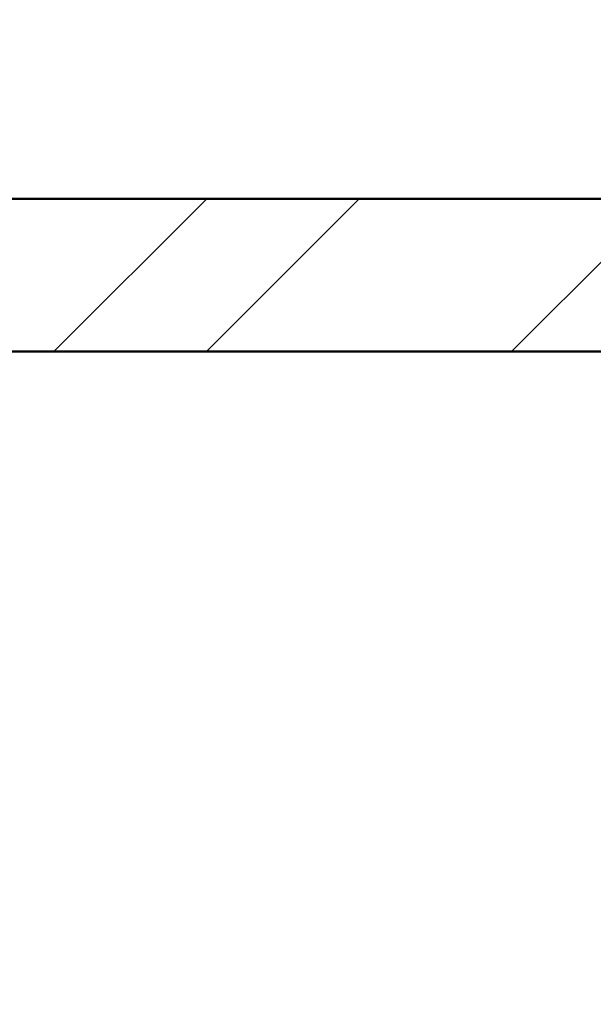
# Model space of a CAD drawing. Units: inches. Extents: x 1901 to 2863, y 888 to 2433.
# Tile 27 of 91: x 2540 to 2557, y 1376 to 1405. Entities that reach past the tile are written whole.
import ezdxf

# ---------------------------------------------------------------- set-up
doc = ezdxf.new("R2010")
doc.units = ezdxf.units.IN
doc.layers.add('A-WALL', color=7, linetype='Continuous', lineweight=50)
doc.layers.add('A-WALL-PATT', color=8, linetype='Continuous', lineweight=13)

msp = doc.modelspace()

# ---------------------------------------------------------------- hatches: boundary and pattern name
at = {"layer": 'A-WALL-PATT'}
h = msp.add_hatch(dxfattribs=at)
h.set_pattern_fill('ANSI32', color=256)
h.paths.add_polyline_path([(2443.926, 2139.888), (2439.426, 2139.888), (2439.426, 2069.348), (2441.676, 2069.348), (2443.926, 2069.348), (2443.926, 2078.634), (2521.926, 2078.634), (2521.926, 2075.067), (2524.176, 2075.067), (2526.426, 2075.067), (2526.426, 2078.634), (2571.755, 2078.634), (2571.755, 2080.884), (2571.755, 2083.134), (2443.926, 2083.134)])
h.paths.add_polyline_path([(2526.426, 2054.634), (2524.176, 2054.634), (2521.926, 2054.634), (2521.926, 2030.634), (2443.926, 2030.634), (2443.926, 2045.348), (2439.426, 2045.348), (2439.426, 1983.867), (2443.926, 1983.867), (2443.926, 2026.134), (2521.926, 2026.134), (2526.426, 2026.134)])
h.paths.add_polyline_path([(2443.926, 1923.867), (2439.426, 1923.867), (2439.426, 1872.634), (2443.926, 1872.634)])
h.paths.add_polyline_path([(2636.233, 1766.134), (2609.926, 1766.134), (2609.926, 1779.785), (2605.426, 1779.785), (2605.426, 1766.134), (2486.614, 1766.134), (2486.614, 1770.671), (2482.114, 1770.671), (2482.114, 1766.134), (2482.114, 1761.634), (2636.233, 1761.634), (2636.233, 1763.884)])
h.paths.add_polyline_path([(2519.536, 1663.384), (2519.536, 1665.634), (2494.926, 1665.634), (2481.831, 1665.634), (2481.831, 1663.384), (2481.831, 1661.134), (2490.426, 1661.134), (2490.426, 1640.157), (2494.926, 1640.157), (2494.926, 1661.134), (2519.536, 1661.134)])
h.paths.add_polyline_path([(2443.926, 1712.134), (2443.926, 1716.634), (2414.464, 1716.634), (2414.464, 1712.134), (2439.426, 1712.134), (2439.426, 1545.507), (2443.926, 1545.507), (2443.926, 1661.134), (2448.475, 1661.134), (2448.475, 1665.634), (2443.926, 1665.634)])
h.paths.add_polyline_path([(2343.426, 1712.134), (2365.525, 1712.134), (2365.525, 1714.384), (2365.525, 1716.634), (2333.871, 1716.634), (2333.871, 1714.384), (2333.871, 1712.134), (2338.926, 1712.134), (2338.926, 1575.634), (2338.926, 1545.507), (2343.426, 1545.507), (2343.426, 1547.507), (2343.426, 1580.134)])
h.paths.add_polyline_path([(2752.926, 1665.634), (2579.536, 1665.634), (2579.536, 1661.134), (2615.926, 1661.134), (2615.926, 1529.134), (2598.931, 1529.134), (2598.931, 1524.634), (2623.127, 1524.634), (2623.127, 1526.884), (2623.127, 1529.134), (2620.426, 1529.134), (2620.426, 1661.134), (2748.426, 1661.134), (2748.426, 1633.499), (2752.926, 1633.499)])
h.paths.add_polyline_path([(2752.926, 1419.929), (2748.426, 1419.929), (2748.426, 1400.134), (2659.426, 1400.134), (2659.426, 1444.333), (2657.176, 1444.333), (2654.926, 1444.333), (2654.926, 1400.134), (2643.649, 1400.134), (2643.649, 1395.634), (2748.426, 1395.634), (2748.426, 1364.035), (2752.926, 1364.035)])
h.paths.add_polyline_path([(2752.926, 1492.878), (2748.426, 1492.878), (2748.426, 1476.634), (2667.426, 1476.634), (2667.426, 1479.71), (2665.176, 1479.71), (2662.926, 1479.71), (2662.926, 1476.634), (2654.926, 1476.634), (2654.926, 1469.536), (2659.426, 1469.536), (2659.426, 1472.134), (2748.426, 1472.134), (2748.426, 1455.929), (2752.926, 1455.929)])
h.paths.add_polyline_path([(2752.926, 1304.035), (2748.426, 1304.035), (2748.426, 1263.634), (2738.66, 1263.634), (2738.66, 1259.134), (2752.926, 1259.134)])
h.paths.add_polyline_path([(2685.926, 1259.134), (2695.49, 1259.134), (2695.49, 1261.384), (2695.49, 1263.634), (2677.837, 1263.634), (2677.837, 1261.384), (2677.837, 1259.134), (2681.426, 1259.134), (2681.426, 1203.634), (2653.277, 1203.634), (2653.277, 1199.134), (2685.926, 1199.134), (2685.926, 1203.634)])
h.paths.add_polyline_path([(2609.426, 1395.634), (2611.848, 1395.634), (2611.848, 1400.134), (2598.888, 1400.134), (2598.888, 1397.884), (2598.888, 1395.634), (2604.926, 1395.634), (2604.926, 1268.134), (2554.726, 1268.134), (2554.726, 1265.884), (2554.726, 1263.634), (2604.926, 1263.634), (2604.926, 1203.634), (2571.306, 1203.634), (2571.306, 1199.134), (2604.926, 1199.134), (2629.277, 1199.134), (2629.277, 1201.384), (2629.277, 1203.634), (2609.426, 1203.634), (2609.426, 1258.634), (2609.426, 1259.134), (2654.804, 1259.134), (2654.804, 1263.634), (2609.426, 1263.634)])
h.paths.add_polyline_path([(2443.926, 1304.035), (2439.426, 1304.035), (2439.426, 1259.134), (2443.926, 1259.134), (2456.16, 1259.134), (2456.16, 1261.384), (2456.16, 1263.634), (2443.926, 1263.634)])
h.paths.add_polyline_path([(2525.426, 1263.634), (2531.778, 1263.634), (2531.778, 1268.134), (2520.926, 1268.134), (2520.926, 1263.634), (2511.409, 1263.634), (2511.409, 1259.134), (2520.926, 1259.134), (2520.926, 1199.134), (2547.306, 1199.134), (2547.306, 1201.384), (2547.306, 1203.634), (2525.426, 1203.634)])
h.paths.add_polyline_path([(2443.926, 1434.842), (2439.426, 1434.842), (2439.426, 1364.035), (2441.676, 1364.035), (2443.926, 1364.035)])
h.paths.add_polyline_path([(2567.134, 1400.134), (2443.926, 1400.134), (2443.926, 1395.634), (2567.134, 1395.634)])
h.paths.add_polyline_path([(2443.926, 1545.507), (2439.426, 1545.507), (2439.426, 1494.842), (2443.926, 1494.842)])
h.paths.add_polyline_path([(2494.926, 1553.349), (2492.676, 1553.349), (2490.426, 1553.349), (2490.426, 1524.634), (2494.926, 1524.634), (2525.936, 1524.634), (2525.936, 1526.884), (2525.936, 1529.134), (2494.926, 1529.134)])
h.paths.add_polyline_path([(2752.926, 1573.499), (2748.426, 1573.499), (2748.426, 1529.134), (2657.759, 1529.134), (2657.759, 1524.634), (2662.926, 1524.634), (2662.926, 1498.631), (2667.426, 1498.631), (2667.426, 1524.634), (2748.426, 1524.634), (2748.426, 1516.878), (2752.926, 1516.878)])
h.paths.add_polyline_path([(2038.602, 2237.418), (2080.174, 2237.418), (2080.174, 2256.075), (2038.602, 2256.075)], flags=9)
h.paths.add_polyline_path([(2292.009, 1062.394), (2539.932, 1062.394), (2539.932, 1099.487), (2292.009, 1099.487)], flags=9)
h.paths.add_polyline_path([(2424.91, 1832.253), (2448.513, 1832.253), (2448.513, 1846.678), (2424.91, 1846.678)], flags=9)
h.paths.add_polyline_path([(2359.076, 1832.253), (2382.678, 1832.253), (2382.678, 1846.678), (2359.076, 1846.678)], flags=9)
h.paths.add_polyline_path([(2352.899, 1684.802), (2367.543, 1684.802), (2367.543, 1697.167), (2352.899, 1697.167)], flags=9)
h.paths.add_polyline_path([(2079.288, 1755.826), (2169.024, 1755.826), (2169.024, 1774.372), (2079.288, 1774.372)], flags=9)
h.paths.add_polyline_path([(2404.09, 1373.857), (2404.09, 1463.593), (2385.544, 1463.593), (2385.544, 1373.857)], flags=9)
h.paths.add_polyline_path([(2268.091, 2236.371), (2309.636, 2236.371), (2309.636, 2255.028), (2268.091, 2255.028)], flags=9)
h.paths.add_polyline_path([(2575.96, 1700.951), (2665.696, 1700.951), (2665.696, 1719.498), (2575.96, 1719.498)], flags=9)
h.paths.add_polyline_path([(2302.962, 1878.474), (2329.524, 1878.474), (2329.524, 1888.777), (2302.962, 1888.777)], flags=9)
h.paths.add_polyline_path([(2097.415, 2240.576), (2126.573, 2240.576), (2126.573, 2259.233), (2097.415, 2259.233)], flags=9)
h.paths.add_polyline_path([(2208.725, 2246.124), (2237.882, 2246.124), (2237.882, 2264.781), (2208.725, 2264.781)], flags=9)
h.paths.add_polyline_path([(2038.147, 1925.958), (2076.987, 1925.958), (2076.987, 1944.615), (2038.147, 1944.615)], flags=9)
h.paths.add_polyline_path([(2239.144, 1926.672), (2288.465, 1926.672), (2288.465, 1945.329), (2239.144, 1945.329)], flags=9)
h.paths.add_polyline_path([(2175.429, 2007.33), (2212.356, 2007.33), (2212.356, 2025.987), (2175.429, 2025.987)], flags=9)
h.paths.add_polyline_path([(2225.034, 2091.794), (2263.875, 2091.794), (2263.875, 2110.451), (2225.034, 2110.451)], flags=9)
h.paths.add_polyline_path([(2035.398, 2098.478), (2074.238, 2098.478), (2074.238, 2117.135), (2035.398, 2117.135)], flags=9)
h.paths.add_polyline_path([(2050.102, 2029.209), (2083.26, 2029.209), (2083.26, 2047.866), (2050.102, 2047.866)], flags=9)
h.paths.add_polyline_path([(2069.677, 1956.719), (2098.835, 1956.719), (2098.835, 1975.376), (2069.677, 1975.376)], flags=9)
h.paths.add_polyline_path([(2328.62, 1753.336), (2361.663, 1753.336), (2361.663, 1771.993), (2328.62, 1771.993)], flags=9)
h.paths.add_polyline_path([(2395.162, 2060.888), (2395.162, 2140.654), (2378.676, 2140.654), (2378.676, 2060.888)], flags=9)
h.paths.add_polyline_path([(2463.728, 2059.02), (2492.886, 2059.02), (2492.886, 2077.677), (2463.728, 2077.677)], flags=9)
h.paths.add_polyline_path([(2458.027, 2181.536), (2496.868, 2181.536), (2496.868, 2200.194), (2458.027, 2200.194)], flags=9)
h.paths.add_polyline_path([(2456.855, 2228.831), (2498.401, 2228.831), (2498.401, 2247.488), (2456.855, 2247.488)], flags=9)
h.paths.add_polyline_path([(2527.577, 2243.074), (2556.735, 2243.074), (2556.735, 2261.731), (2527.577, 2261.731)], flags=9)
h.paths.add_polyline_path([(2694.461, 2232.767), (2736.033, 2232.767), (2736.033, 2251.425), (2694.461, 2251.425)], flags=9)
h.paths.add_polyline_path([(2637.821, 2249.225), (2666.979, 2249.225), (2666.979, 2267.882), (2637.821, 2267.882)], flags=9)
h.paths.add_polyline_path([(2623.687, 2183.541), (2662.528, 2183.541), (2662.528, 2202.199), (2623.687, 2202.199)], flags=9)
h.paths.add_polyline_path([(2691.965, 2021.5), (2725.124, 2021.5), (2725.124, 2040.157), (2691.965, 2040.157)], flags=9)
h.paths.add_polyline_path([(2621.043, 1975.912), (2662.335, 1975.912), (2662.335, 1994.569), (2621.043, 1994.569)], flags=9)
h.paths.add_polyline_path([(2479.032, 1927.62), (2519.844, 1927.62), (2519.844, 1946.277), (2479.032, 1946.277)], flags=9)
h.paths.add_polyline_path([(2670.941, 1849.076), (2716.005, 1849.076), (2716.005, 1867.734), (2670.941, 1867.734)], flags=9)
h.paths.add_polyline_path([(2523.613, 1782.956), (2550.175, 1782.956), (2550.175, 1793.26), (2523.613, 1793.26)], flags=9)
h.paths.add_polyline_path([(2450.841, 1207.331), (2492.386, 1207.331), (2492.386, 1225.989), (2450.841, 1225.989)], flags=9)
h.paths.add_polyline_path([(2527.751, 1203.841), (2556.908, 1203.841), (2556.908, 1222.499), (2527.751, 1222.499)], flags=9)
h.paths.add_polyline_path([(2639.111, 1207.2), (2668.268, 1207.2), (2668.268, 1225.857), (2639.111, 1225.857)], flags=9)
h.paths.add_polyline_path([(2692.594, 1218.965), (2734.167, 1218.965), (2734.167, 1237.623), (2692.594, 1237.623)], flags=9)
h.paths.add_polyline_path([(2669.266, 1366.329), (2708.106, 1366.329), (2708.106, 1384.987), (2669.266, 1384.987)], flags=25)
h.paths.add_polyline_path([(2463.313, 1358.031), (2502.153, 1358.031), (2502.153, 1376.688), (2463.313, 1376.688)], flags=9)
h.paths.add_polyline_path([(2494.725, 1449.963), (2531.652, 1449.963), (2531.652, 1468.62), (2494.725, 1468.62)], flags=9)
h.paths.add_polyline_path([(2675.565, 1422.157), (2708.724, 1422.157), (2708.724, 1440.815), (2675.565, 1440.815)], flags=25)
h.paths.add_polyline_path([(2685.634, 1493.891), (2714.792, 1493.891), (2714.792, 1512.548), (2685.634, 1512.548)], flags=9)
h.paths.add_polyline_path([(2686.805, 1529.913), (2725.645, 1529.913), (2725.645, 1548.57), (2686.805, 1548.57)], flags=25)
h.paths.add_polyline_path([(2503.651, 1537.991), (2552.972, 1537.991), (2552.972, 1556.648), (2503.651, 1556.648)], flags=9)
h.paths.add_polyline_path([(2291.713, 1643.504), (2318.275, 1643.504), (2318.275, 1653.807), (2291.713, 1653.807)], flags=9)
h.paths.add_polyline_path([(2450.626, 1610.52), (2477.189, 1610.52), (2477.189, 1620.824), (2450.626, 1620.824)], flags=9)
h.paths.add_polyline_path([(2359.985, 1551.814), (2422.253, 1551.814), (2422.253, 1562.117), (2359.985, 1562.117)], flags=9)
h.paths.add_polyline_path([(2280.106, 1249.006), (2321.651, 1249.006), (2321.651, 1267.663), (2280.106, 1267.663)], flags=9)
h.paths.add_polyline_path([(2164.057, 1274.232), (2193.215, 1274.232), (2193.215, 1292.889), (2164.057, 1292.889)], flags=9)
h.paths.add_polyline_path([(2118.21, 1277.694), (2151.252, 1277.694), (2151.252, 1296.351), (2118.21, 1296.351)], flags=9)
h.paths.add_polyline_path([(2031.946, 1268.529), (2073.519, 1268.529), (2073.519, 1287.187), (2031.946, 1287.187)], flags=9)
h.paths.add_polyline_path([(2050.199, 1409.079), (2089.04, 1409.079), (2089.04, 1427.736), (2050.199, 1427.736)], flags=9)
h.paths.add_polyline_path([(2243.743, 1421.032), (2282.584, 1421.032), (2282.584, 1439.689), (2243.743, 1439.689)], flags=9)
h.paths.add_polyline_path([(2190.746, 1509.769), (2231.558, 1509.769), (2231.558, 1528.426), (2190.746, 1528.426)], flags=9)
h.paths.add_polyline_path([(2058.392, 1475.415), (2091.55, 1475.415), (2091.55, 1494.073), (2058.392, 1494.073)], flags=9)
h.paths.add_polyline_path([(2062.447, 1553.09), (2091.605, 1553.09), (2091.605, 1571.747), (2062.447, 1571.747)], flags=9)
h.paths.add_polyline_path([(2219.524, 1590.365), (2266.147, 1590.365), (2266.147, 1609.022), (2219.524, 1609.022)], flags=9)
h.paths.add_polyline_path([(2041.072, 1584.188), (2079.912, 1584.188), (2079.912, 1602.845), (2041.072, 1602.845)], flags=9)

# ---------------------------------------------------------------- linework, layer by layer
at = {"layer": 'A-WALL'}
for p, q in [((2443.926, 1400.134), (2567.134, 1400.134)), ((2443.926, 1395.634), (2568.638, 1395.634))]:
    msp.add_line(p, q, dxfattribs=at)

doc.saveas('drawing.dxf')
